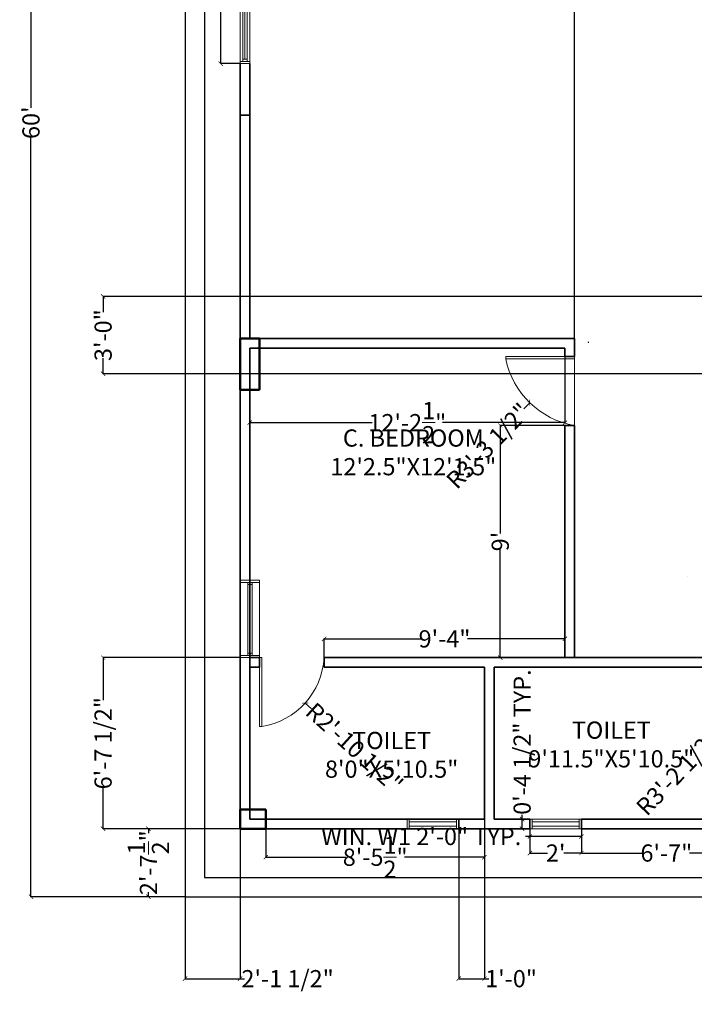
# Model space of a CAD drawing. Units: inches. Extents: x 490 to 1091, y 501 to 1322.
# Tile 1 of 5: x 490 to 804, y 501 to 959. Entities that reach past the tile are written whole.
import ezdxf

# ---------------------------------------------------------------- set-up
doc = ezdxf.new("R2010")
doc.units = ezdxf.units.IN
doc.header["$MEASUREMENT"] = 0
doc.linetypes.add('ACAD_ISO02W100', pattern=[15, 12, -3])
for name, color, linetype, lineweight in [('A-ANNO-DIMS', 2, 'Continuous', 18), ('A-ANNO-REFR', 8, 'Continuous', 13), ('A-AREA-IDEN', 7, 'Continuous', 25), ('A-COLS', 12, 'Continuous', 50), ('A-DOOR', 3, 'Continuous', 20), ('A-GLAZ', 4, 'Continuous', 18), ('A-WALL', 7, 'Continuous', 35), ('A-WALL-HIDN', 7, 'ACAD_ISO02W100', 18), ('C-PROP', 8, 'Continuous', 25)]:
    doc.layers.add(name, color=color, linetype=linetype, lineweight=lineweight)
doc.styles.get("Standard").update_dxf_attribs({"font": 'arial.ttf'})
doc.dimstyles.get("Standard").update_dxf_attribs({"dimtxt": 8, "dimasz": 2, "dimexe": 0.18, "dimexo": 0.0625, "dimgap": 0.09, "dimtad": 0, "dimdec": 1, "dimzin": 0, "dimdsep": 46, "dimlunit": 4, "dimtxsty": 'Standard', "dimblk": 'ARCHTICK', "dimcen": 0.09, "dimadec": 0, "dimazin": 0, "dimtfac": 1, "dimtdec": 1, "dimtofl": 0, "dimtmove": 0, "dimatfit": 3, "dimldrblk": 'ARCHTICK', "dimfxl": 1, "dimtolj": 1, "dimtzin": 0, "dimarcsym": 0})

# ---------------------------------------------------------------- blocks, each defined once
blk = doc.blocks.new('_ArchTick')
at = {"color": 0, "linetype": 'ByBlock', "const_width": 0.15}
blk.add_lwpolyline([(-0.5, -0.5), (0.5, 0.5)], dxfattribs=at)
blk = doc.blocks.new('*D4')
at = {"layer": 'A-ANNO-DIMS', "color": 0, "lineweight": -2, "transparency": 16777216}
for p, q in [((567.21, 1270.88), (495.41, 1270.88)), ((495.59, 1270.88), (495.59, 917.79)), ((495.59, 550.88), (495.59, 903.98)), ((567.21, 550.88), (495.41, 550.88))]:
    blk.add_line(p, q, dxfattribs=at)
at = {"layer": 'Defpoints', "color": 0, "transparency": 16777216}
for p in [(567.27, 1270.88), (495.59, 550.88), (567.27, 550.88)]:
    blk.add_point(p, dxfattribs=at)
at = {"layer": 'A-ANNO-DIMS', "color": 0, "lineweight": -2, "transparency": 16777216, "xscale": 2, "yscale": 2, "zscale": 2}
for p, rotation in [((495.59, 1270.88), 90), ((495.59, 550.88), 270)]:
    blk.add_blockref('_ArchTick', p, dxfattribs=dict(at, rotation=rotation))
at = {"layer": 'A-ANNO-DIMS', "color": 0, "transparency": 16777216, "insert": (495.59, 910.88), "char_height": 8, "attachment_point": 5, "rotation": 90}
blk.add_mtext("\\A1;60'", dxfattribs=at)
blk = doc.blocks.new('bfgbfhnfh')
for p, q in [((1236.93, 946.75), (1241.43, 946.75)), ((1236.93, 922.75), (1236.93, 946.75)), ((1236.93, 945.75), (1241.43, 945.75)), ((1238.18, 945.75), (1238.18, 923.75)), ((1240.18, 945.75), (1240.18, 923.75)), ((1241.43, 946.75), (1241.43, 922.75)), ((1241.43, 923.75), (1236.93, 923.75)), ((1241.43, 922.75), (1236.93, 922.75))]:
    blk.add_line(p, q)
blk = doc.blocks.new('bnfgfhvhm')
for p, q in [((1106.43, 1203.63), (1115.43, 1203.63)), ((1106.43, 1191.63), (1106.43, 1203.63)), ((1115.43, 1203.63), (1115.43, 1191.63)), ((1115.43, 1191.63), (1106.43, 1191.63))]:
    blk.add_line(p, q)
blk = doc.blocks.new('*D18')
at = {"layer": 'A-ANNO-DIMS', "color": 0, "lineweight": -2, "transparency": 16777216}
for p, q in [((751.67, 586.92), (751.67, 571.01)), ((830.67, 586.92), (830.67, 571.01)), ((751.67, 571.19), (780.42, 571.19)), ((830.67, 571.19), (801.91, 571.19))]:
    blk.add_line(p, q, dxfattribs=at)
at = {"layer": 'Defpoints', "color": 0, "transparency": 16777216}
for p in [(751.67, 586.98), (830.67, 586.98), (751.67, 571.19)]:
    blk.add_point(p, dxfattribs=at)
at = {"layer": 'A-ANNO-DIMS', "color": 0, "lineweight": -2, "transparency": 16777216, "xscale": 2, "yscale": 2, "zscale": 2, "rotation": 180}
blk.add_blockref('_ArchTick', (751.67, 571.19), dxfattribs=at)
at = {"layer": 'A-ANNO-DIMS', "color": 0, "lineweight": -2, "transparency": 16777216, "xscale": 2, "yscale": 2, "zscale": 2}
blk.add_blockref('_ArchTick', (830.67, 571.19), dxfattribs=at)
at = {"layer": 'A-ANNO-DIMS', "color": 0, "transparency": 16777216, "insert": (791.17, 571.19), "char_height": 8, "attachment_point": 5}
blk.add_mtext('\\A1;6\'-7"', dxfattribs=at)
blk = doc.blocks.new('*D19')
at = {"layer": 'A-ANNO-DIMS', "color": 0, "lineweight": -2, "transparency": 16777216}
for p, q in [((727.67, 582.42), (727.67, 571.01)), ((751.67, 582.42), (751.67, 571.01)), ((727.67, 571.19), (735.83, 571.19)), ((751.67, 571.19), (743.51, 571.19))]:
    blk.add_line(p, q, dxfattribs=at)
at = {"layer": 'Defpoints', "color": 0, "transparency": 16777216}
for p in [(727.67, 582.48), (751.67, 582.48), (751.67, 571.19)]:
    blk.add_point(p, dxfattribs=at)
at = {"layer": 'A-ANNO-DIMS', "color": 0, "lineweight": -2, "transparency": 16777216, "xscale": 2, "yscale": 2, "zscale": 2, "rotation": 180}
blk.add_blockref('_ArchTick', (727.67, 571.19), dxfattribs=at)
at = {"layer": 'A-ANNO-DIMS', "color": 0, "lineweight": -2, "transparency": 16777216, "xscale": 2, "yscale": 2, "zscale": 2}
blk.add_blockref('_ArchTick', (751.67, 571.19), dxfattribs=at)
at = {"layer": 'A-ANNO-DIMS', "color": 0, "transparency": 16777216, "insert": (739.67, 571.19), "char_height": 8, "attachment_point": 5}
blk.add_mtext("\\A1;2'", dxfattribs=at)
blk = doc.blocks.new('*D20')
at = {"layer": 'A-ANNO-DIMS', "color": 0, "lineweight": -2, "transparency": 16777216}
for p, q in [((604.87, 586.92), (604.87, 569.06)), ((706.57, 586.92), (706.57, 569.06)), ((604.87, 569.24), (642.07, 569.24)), ((706.57, 569.24), (669.37, 569.24))]:
    blk.add_line(p, q, dxfattribs=at)
at = {"layer": 'Defpoints', "color": 0, "transparency": 16777216}
for p in [(604.87, 586.98), (706.57, 586.98), (706.57, 569.24)]:
    blk.add_point(p, dxfattribs=at)
at = {"layer": 'A-ANNO-DIMS', "color": 0, "lineweight": -2, "transparency": 16777216, "xscale": 2, "yscale": 2, "zscale": 2, "rotation": 180}
blk.add_blockref('_ArchTick', (604.87, 569.24), dxfattribs=at)
at = {"layer": 'A-ANNO-DIMS', "color": 0, "lineweight": -2, "transparency": 16777216, "xscale": 2, "yscale": 2, "zscale": 2}
blk.add_blockref('_ArchTick', (706.57, 569.24), dxfattribs=at)
at = {"layer": 'A-ANNO-DIMS', "color": 0, "transparency": 16777216, "insert": (655.72, 569.24), "char_height": 8, "attachment_point": 5}
blk.add_mtext('\\A1;8\'-5{\\H1x;\\S1/2;}"', dxfattribs=at)
blk = doc.blocks.new('*D21')
at = {"layer": 'A-ANNO-DIMS', "color": 0, "lineweight": -2, "transparency": 16777216}
for p, q in [((631.97, 662.15), (631.97, 670.99)), ((631.97, 670.81), (677.25, 670.81)), ((743.97, 670.81), (698.69, 670.81)), ((743.97, 662.15), (743.97, 670.99))]:
    blk.add_line(p, q, dxfattribs=at)
at = {"layer": 'Defpoints', "color": 0, "transparency": 16777216}
for p in [(631.97, 670.81), (631.97, 662.08), (743.97, 662.08)]:
    blk.add_point(p, dxfattribs=at)
at = {"layer": 'A-ANNO-DIMS', "color": 0, "lineweight": -2, "transparency": 16777216, "xscale": 2, "yscale": 2, "zscale": 2, "rotation": 180}
blk.add_blockref('_ArchTick', (631.97, 670.81), dxfattribs=at)
at = {"layer": 'A-ANNO-DIMS', "color": 0, "lineweight": -2, "transparency": 16777216, "xscale": 2, "yscale": 2, "zscale": 2}
blk.add_blockref('_ArchTick', (743.97, 670.81), dxfattribs=at)
at = {"layer": 'A-ANNO-DIMS', "color": 0, "transparency": 16777216, "insert": (687.97, 670.81), "char_height": 8, "attachment_point": 5}
blk.add_mtext('\\A1;9\'-4"', dxfattribs=at)
blk = doc.blocks.new('ggnhgjgfjhgjjjjjjjj')
for p, q in [((597.37, 998.37), (592.87, 998.37)), ((592.87, 998.37), (592.87, 938.37)), ((597.37, 998.37), (592.87, 998.37)), ((597.37, 997.37), (592.87, 997.37)), ((594.12, 997.37), (594.12, 939.37)), ((596.12, 996.37), (594.12, 996.37)), ((595.12, 996.37), (595.12, 940.37)), ((596.12, 997.37), (596.12, 939.37)), ((597.37, 938.37), (597.37, 998.37)), ((592.87, 939.37), (597.37, 939.37)), ((594.12, 940.37), (596.12, 940.37)), ((597.37, 938.37), (592.87, 938.37)), ((592.87, 938.37), (597.37, 938.37))]:
    blk.add_line(p, q)
blk = doc.blocks.new('jcjg  bmvh')
for p, q in [((1232.66, 1066.6), (1223.66, 1066.6)), ((1223.66, 1066.6), (1223.66, 1042.6)), ((1232.66, 1042.6), (1232.66, 1066.6)), ((1223.66, 1042.6), (1232.66, 1042.6))]:
    blk.add_line(p, q)
blk = doc.blocks.new('fvbfbvc hbmh')
for p, q in [((1342.5, 1176.65), (1378.5, 1176.65)), ((1342.5, 1167.65), (1342.5, 1176.65)), ((1343.5, 1167.65), (1343.5, 1176.65)), ((1343.5, 1173.15), (1377.5, 1173.15)), ((1344.5, 1171.15), (1344.5, 1173.15)), ((1376.5, 1173.15), (1376.5, 1171.15)), ((1377.5, 1176.65), (1377.5, 1167.65)), ((1378.5, 1176.65), (1378.5, 1167.65)), ((1343.5, 1171.15), (1377.5, 1171.15)), ((1344.5, 1172.15), (1376.5, 1172.15)), ((1378.5, 1167.65), (1342.5, 1167.65))]:
    blk.add_line(p, q)
blk = doc.blocks.new('*D36')
at = {"layer": 'A-ANNO-DIMS', "color": 0, "lineweight": -2, "transparency": 16777216}
for p, q in [((592.81, 582.48), (550.06, 582.48)), ((550.24, 582.48), (550.24, 580.39)), ((567.21, 550.88), (550.06, 550.88)), ((550.24, 550.88), (550.24, 552.98))]:
    blk.add_line(p, q, dxfattribs=at)
at = {"layer": 'Defpoints', "color": 0, "transparency": 16777216}
for p in [(550.24, 582.48), (592.87, 582.48), (567.27, 550.88)]:
    blk.add_point(p, dxfattribs=at)
at = {"layer": 'A-ANNO-DIMS', "color": 0, "lineweight": -2, "transparency": 16777216, "xscale": 2, "yscale": 2, "zscale": 2}
for p, rotation in [((550.24, 582.48), 90), ((550.24, 550.88), 270)]:
    blk.add_blockref('_ArchTick', p, dxfattribs=dict(at, rotation=rotation))
at = {"layer": 'A-ANNO-DIMS', "color": 0, "transparency": 16777216, "insert": (550.24, 566.68), "char_height": 8, "attachment_point": 5, "rotation": 90}
blk.add_mtext('\\A1;2\'-7{\\H1x;\\S1/2;}"', dxfattribs=at)
blk = doc.blocks.new('*D38')
at = {"layer": 'A-ANNO-DIMS', "color": 0, "lineweight": -2, "transparency": 16777216}
for p, q in [((748.41, 770.08), (713.71, 770.08)), ((713.89, 770.08), (713.89, 719.86)), ((713.89, 662.08), (713.89, 712.31)), ((748.41, 662.08), (713.71, 662.08))]:
    blk.add_line(p, q, dxfattribs=at)
at = {"layer": 'Defpoints', "color": 0, "transparency": 16777216}
for p in [(748.47, 770.08), (713.89, 662.08), (748.47, 662.08)]:
    blk.add_point(p, dxfattribs=at)
at = {"layer": 'A-ANNO-DIMS', "color": 0, "lineweight": -2, "transparency": 16777216, "xscale": 2, "yscale": 2, "zscale": 2}
for p, rotation in [((713.89, 770.08), 90), ((713.89, 662.08), 270)]:
    blk.add_blockref('_ArchTick', p, dxfattribs=dict(at, rotation=rotation))
at = {"layer": 'A-ANNO-DIMS', "color": 0, "transparency": 16777216, "insert": (713.89, 716.08), "char_height": 8, "attachment_point": 5, "rotation": 90}
blk.add_mtext("\\A1;9'", dxfattribs=at)
blk = doc.blocks.new('*D39')
at = {"layer": 'A-ANNO-DIMS', "color": 0, "lineweight": -2, "transparency": 16777216}
for p, q in [((597.37, 806.02), (597.37, 771.19)), ((743.97, 806.02), (743.97, 771.19)), ((597.37, 771.37), (654.3, 771.37)), ((743.97, 771.37), (687.04, 771.37))]:
    blk.add_line(p, q, dxfattribs=at)
at = {"layer": 'Defpoints', "color": 0, "transparency": 16777216}
for p in [(597.37, 806.08), (743.97, 806.08), (743.97, 771.37)]:
    blk.add_point(p, dxfattribs=at)
at = {"layer": 'A-ANNO-DIMS', "color": 0, "lineweight": -2, "transparency": 16777216, "xscale": 2, "yscale": 2, "zscale": 2, "rotation": 180}
blk.add_blockref('_ArchTick', (597.37, 771.37), dxfattribs=at)
at = {"layer": 'A-ANNO-DIMS', "color": 0, "lineweight": -2, "transparency": 16777216, "xscale": 2, "yscale": 2, "zscale": 2}
blk.add_blockref('_ArchTick', (743.97, 771.37), dxfattribs=at)
at = {"layer": 'A-ANNO-DIMS', "color": 0, "transparency": 16777216, "insert": (670.67, 771.37), "char_height": 8, "attachment_point": 5}
blk.add_mtext('\\A1;12\'-2{\\H1x;\\S1/2;}"', dxfattribs=at)
blk = doc.blocks.new('DOOR-LEAF-32IN')
for p, q in [((-32, -1), (-32, 0)), ((-32, 0), (0, 0)), ((0, 0), (0, -1)), ((0, -1), (-32, -1))]:
    blk.add_line(p, q)
blk = doc.blocks.new('*D58')
at = {"layer": 'A-ANNO-DIMS', "color": 0, "lineweight": -2, "transparency": 16777216}
for p, q in [((727.67, 582.42), (727.67, 578.7)), ((751.67, 582.42), (751.67, 578.7)), ((727.67, 578.88), (725.67, 578.88)), ((751.67, 578.88), (727.67, 578.88))]:
    blk.add_line(p, q, dxfattribs=at)
at = {"layer": 'Defpoints', "color": 0, "transparency": 16777216}
for p in [(727.67, 582.48), (751.67, 582.48), (727.67, 578.88)]:
    blk.add_point(p, dxfattribs=at)
at = {"layer": 'A-ANNO-DIMS', "color": 0, "lineweight": -2, "transparency": 16777216, "xscale": 2, "yscale": 2, "zscale": 2, "rotation": 180}
blk.add_blockref('_ArchTick', (727.67, 578.88), dxfattribs=at)
at = {"layer": 'A-ANNO-DIMS', "color": 0, "lineweight": -2, "transparency": 16777216, "xscale": 2, "yscale": 2, "zscale": 2}
blk.add_blockref('_ArchTick', (751.67, 578.88), dxfattribs=at)
at = {"layer": 'A-ANNO-DIMS', "color": 0, "transparency": 16777216, "insert": (677.13, 578.88), "char_height": 8, "attachment_point": 5}
blk.add_mtext('\\A1;WIN. W1 2\'-0" TYP.', dxfattribs=at)
blk = doc.blocks.new('*D59')
at = {"layer": 'A-ANNO-DIMS', "color": 0, "lineweight": -2, "transparency": 16777216}
for p, q in [((727.61, 586.98), (723.89, 586.98)), ((724.07, 586.98), (724.07, 588.98)), ((724.07, 582.48), (724.07, 586.98)), ((727.61, 582.48), (723.89, 582.48))]:
    blk.add_line(p, q, dxfattribs=at)
at = {"layer": 'Defpoints', "color": 0, "transparency": 16777216}
for p in [(724.07, 586.98), (727.67, 586.98), (727.67, 582.48)]:
    blk.add_point(p, dxfattribs=at)
at = {"layer": 'A-ANNO-DIMS', "color": 0, "lineweight": -2, "transparency": 16777216, "xscale": 2, "yscale": 2, "zscale": 2}
for p, rotation in [((724.07, 586.98), 90), ((724.07, 582.48), 270)]:
    blk.add_blockref('_ArchTick', p, dxfattribs=dict(at, rotation=rotation))
at = {"layer": 'A-ANNO-DIMS', "color": 0, "transparency": 16777216, "insert": (724.07, 622.78), "char_height": 8, "attachment_point": 5, "rotation": 90}
blk.add_mtext('\\A1;0\'-4 1/2" TYP.', dxfattribs=at)
blk = doc.blocks.new('*D62')
at = {"layer": 'A-ANNO-DIMS', "color": 0, "lineweight": -2, "transparency": 16777216}
for p, q in [((583.87, 998.37), (583.87, 1000.37)), ((592.81, 998.37), (583.69, 998.37)), ((583.87, 938.37), (583.87, 998.37)), ((592.81, 938.37), (583.69, 938.37))]:
    blk.add_line(p, q, dxfattribs=at)
at = {"layer": 'Defpoints', "color": 0, "transparency": 16777216}
for p in [(583.87, 998.37), (592.87, 998.37), (592.87, 938.37)]:
    blk.add_point(p, dxfattribs=at)
at = {"layer": 'A-ANNO-DIMS', "color": 0, "lineweight": -2, "transparency": 16777216, "xscale": 2, "yscale": 2, "zscale": 2}
for p, rotation in [((583.87, 998.37), 90), ((583.87, 938.37), 270)]:
    blk.add_blockref('_ArchTick', p, dxfattribs=dict(at, rotation=rotation))
at = {"layer": 'A-ANNO-DIMS', "color": 0, "transparency": 16777216, "insert": (583.87, 1035.16), "char_height": 8, "attachment_point": 5, "rotation": 90}
blk.add_mtext('\\A1;WIN. W3 5\'-0"', dxfattribs=at)
blk = doc.blocks.new('*D66')
at = {"layer": 'A-ANNO-DIMS', "color": 0, "lineweight": -2, "transparency": 16777216}
for p, q in [((592.87, 582.42), (592.87, 512.57)), ((567.27, 550.82), (567.27, 512.57)), ((567.27, 512.75), (592.87, 512.75)), ((592.87, 512.75), (594.87, 512.75))]:
    blk.add_line(p, q, dxfattribs=at)
at = {"layer": 'Defpoints', "color": 0, "transparency": 16777216}
for p in [(592.87, 582.48), (567.27, 550.88), (592.87, 512.75)]:
    blk.add_point(p, dxfattribs=at)
at = {"layer": 'A-ANNO-DIMS', "color": 0, "lineweight": -2, "transparency": 16777216, "xscale": 2, "yscale": 2, "zscale": 2, "rotation": 180}
blk.add_blockref('_ArchTick', (567.27, 512.75), dxfattribs=at)
at = {"layer": 'A-ANNO-DIMS', "color": 0, "lineweight": -2, "transparency": 16777216, "xscale": 2, "yscale": 2, "zscale": 2}
blk.add_blockref('_ArchTick', (592.87, 512.75), dxfattribs=at)
at = {"layer": 'A-ANNO-DIMS', "color": 0, "transparency": 16777216, "insert": (614.98, 512.75), "char_height": 8, "attachment_point": 5}
blk.add_mtext('\\A1;2\'-1 1/2"', dxfattribs=at)
blk = doc.blocks.new('*D76')
at = {"layer": 'A-ANNO-DIMS', "color": 0, "lineweight": -2, "transparency": 16777216}
for p, q in [((748.47, 802.15), (748.47, 1309.19)), ((748.47, 1309.01), (775.72, 1309.01)), ((830.67, 1309.01), (803.42, 1309.01)), ((830.67, 794.15), (830.67, 1309.19))]:
    blk.add_line(p, q, dxfattribs=at)
at = {"layer": 'Defpoints', "color": 0, "transparency": 16777216}
for p in [(830.67, 1309.01), (748.47, 802.08), (830.67, 794.08)]:
    blk.add_point(p, dxfattribs=at)
at = {"layer": 'A-ANNO-DIMS', "color": 0, "lineweight": -2, "transparency": 16777216, "xscale": 2, "yscale": 2, "zscale": 2, "rotation": 180}
blk.add_blockref('_ArchTick', (748.47, 1309.01), dxfattribs=at)
at = {"layer": 'A-ANNO-DIMS', "color": 0, "lineweight": -2, "transparency": 16777216, "xscale": 2, "yscale": 2, "zscale": 2}
blk.add_blockref('_ArchTick', (830.67, 1309.01), dxfattribs=at)
at = {"layer": 'A-ANNO-DIMS', "color": 0, "transparency": 16777216, "insert": (789.57, 1309.01), "char_height": 8, "attachment_point": 5}
blk.add_mtext('\\A1;6\'-10"', dxfattribs=at)
blk = doc.blocks.new('*D77')
at = {"layer": 'A-ANNO-DIMS', "color": 0, "lineweight": -2, "transparency": 16777216}
for p, q in [((592.91, 662.08), (528.96, 662.08)), ((529.14, 662.08), (529.14, 642.35)), ((529.14, 582.48), (529.14, 602.22)), ((592.81, 582.48), (528.96, 582.48))]:
    blk.add_line(p, q, dxfattribs=at)
at = {"layer": 'Defpoints', "color": 0, "transparency": 16777216}
for p in [(529.14, 662.08), (592.97, 662.08), (592.87, 582.48)]:
    blk.add_point(p, dxfattribs=at)
at = {"layer": 'A-ANNO-DIMS', "color": 0, "lineweight": -2, "transparency": 16777216, "xscale": 2, "yscale": 2, "zscale": 2}
for p, rotation in [((529.14, 662.08), 90), ((529.14, 582.48), 270)]:
    blk.add_blockref('_ArchTick', p, dxfattribs=dict(at, rotation=rotation))
at = {"layer": 'A-ANNO-DIMS', "color": 0, "transparency": 16777216, "insert": (529.14, 622.28), "char_height": 8, "attachment_point": 5, "rotation": 90}
blk.add_mtext('\\A1;6\'-7 1/2"', dxfattribs=at)
blk = doc.blocks.new('*D78')
at = {"layer": 'A-ANNO-DIMS', "color": 0, "lineweight": -2, "transparency": 16777216}
for p, q in [((694.57, 586.92), (694.57, 512.57)), ((706.57, 586.92), (706.57, 512.57)), ((694.57, 512.75), (706.57, 512.75)), ((706.57, 512.75), (708.57, 512.75))]:
    blk.add_line(p, q, dxfattribs=at)
at = {"layer": 'Defpoints', "color": 0, "transparency": 16777216}
for p in [(694.57, 586.98), (706.57, 586.98), (706.57, 512.75)]:
    blk.add_point(p, dxfattribs=at)
at = {"layer": 'A-ANNO-DIMS', "color": 0, "lineweight": -2, "transparency": 16777216, "xscale": 2, "yscale": 2, "zscale": 2, "rotation": 180}
blk.add_blockref('_ArchTick', (694.57, 512.75), dxfattribs=at)
at = {"layer": 'A-ANNO-DIMS', "color": 0, "lineweight": -2, "transparency": 16777216, "xscale": 2, "yscale": 2, "zscale": 2}
blk.add_blockref('_ArchTick', (706.57, 512.75), dxfattribs=at)
at = {"layer": 'A-ANNO-DIMS', "color": 0, "transparency": 16777216, "insert": (718.92, 512.75), "char_height": 8, "attachment_point": 5}
blk.add_mtext('\\A1;1\'-0"', dxfattribs=at)
blk = doc.blocks.new('*D79')
at = {"layer": 'A-ANNO-DIMS', "color": 0, "lineweight": -2, "transparency": 16777216}
for p, q in [((830.61, 830.08), (528.96, 830.08)), ((529.14, 830.08), (529.14, 822.81)), ((529.14, 794.08), (529.14, 801.36)), ((830.61, 794.08), (528.96, 794.08))]:
    blk.add_line(p, q, dxfattribs=at)
at = {"layer": 'Defpoints', "color": 0, "transparency": 16777216}
for p in [(529.14, 830.08), (830.67, 830.08), (830.67, 794.08)]:
    blk.add_point(p, dxfattribs=at)
at = {"layer": 'A-ANNO-DIMS', "color": 0, "lineweight": -2, "transparency": 16777216, "xscale": 2, "yscale": 2, "zscale": 2}
for p, rotation in [((529.14, 830.08), 90), ((529.14, 794.08), 270)]:
    blk.add_blockref('_ArchTick', p, dxfattribs=dict(at, rotation=rotation))
at = {"layer": 'A-ANNO-DIMS', "color": 0, "transparency": 16777216, "insert": (529.14, 812.08), "char_height": 8, "attachment_point": 5, "rotation": 90}
blk.add_mtext('\\A1;3\'-0"', dxfattribs=at)
blk = doc.blocks.new('*D83')
at = {"layer": 'A-ANNO-DIMS', "color": 0, "lineweight": -2, "transparency": 16777216}
for p, q in [((754.87, 808.8), (755.05, 808.8)), ((754.96, 808.71), (754.96, 808.89)), ((724.86, 777.73), (727.64, 780.6))]:
    blk.add_line(p, q, dxfattribs=at)
at = {"layer": 'Defpoints', "color": 0, "transparency": 16777216}
for p in [(754.96, 808.8), (727.64, 780.6)]:
    blk.add_point(p, dxfattribs=at)
at = {"layer": 'A-ANNO-DIMS', "color": 0, "lineweight": -2, "transparency": 16777216, "xscale": 2, "yscale": 2, "zscale": 2, "rotation": 45.90870563316058}
blk.add_blockref('_ArchTick', (727.64, 780.6), dxfattribs=at)
at = {"layer": 'A-ANNO-DIMS', "color": 0, "transparency": 16777216, "insert": (708.25, 760.59), "char_height": 8, "attachment_point": 5, "rotation": 45.9087}
blk.add_mtext('\\A1;R3\'-3 1/2"', dxfattribs=at)
blk = doc.blocks.new('*D84')
at = {"layer": 'A-ANNO-DIMS', "color": 0, "lineweight": -2, "transparency": 16777216}
for p, q in [((842.73, 656.51), (842.91, 656.51)), ((842.82, 656.42), (842.82, 656.6)), ((813.15, 625.82), (815.93, 628.69))]:
    blk.add_line(p, q, dxfattribs=at)
at = {"layer": 'Defpoints', "color": 0, "transparency": 16777216}
for p in [(842.82, 656.51), (815.93, 628.69)]:
    blk.add_point(p, dxfattribs=at)
at = {"layer": 'A-ANNO-DIMS', "color": 0, "lineweight": -2, "transparency": 16777216, "xscale": 2, "yscale": 2, "zscale": 2, "rotation": 45.97167705914391}
blk.add_blockref('_ArchTick', (815.93, 628.69), dxfattribs=at)
at = {"layer": 'A-ANNO-DIMS', "color": 0, "transparency": 16777216, "insert": (796.55, 608.65), "char_height": 8, "attachment_point": 5, "rotation": 45.9717}
blk.add_mtext('\\A1;R3\'-2 1/2"', dxfattribs=at)
blk = doc.blocks.new('*D86')
at = {"layer": 'A-ANNO-DIMS', "color": 0, "lineweight": -2, "transparency": 16777216}
for p, q in [((597.7, 663.91), (597.7, 664.09)), ((597.61, 664), (597.79, 664)), ((626.1, 638.27), (623.13, 640.95))]:
    blk.add_line(p, q, dxfattribs=at)
at = {"layer": 'Defpoints', "color": 0, "transparency": 16777216}
for p in [(597.7, 664), (623.13, 640.95)]:
    blk.add_point(p, dxfattribs=at)
at = {"layer": 'A-ANNO-DIMS', "color": 0, "lineweight": -2, "transparency": 16777216, "xscale": 2, "yscale": 2, "zscale": 2, "rotation": 137.8160408924442}
blk.add_blockref('_ArchTick', (623.13, 640.95), dxfattribs=at)
at = {"layer": 'A-ANNO-DIMS', "color": 0, "transparency": 16777216, "insert": (646.09, 620.15), "char_height": 8, "attachment_point": 5, "rotation": 317.816}
blk.add_mtext('\\A1;R2\'-10 1/2"', dxfattribs=at)

msp = doc.modelspace()

# ---------------------------------------------------------------- linework, layer by layer
at = {"layer": 'A-ANNO-REFR'}
for p, q in [((801.21, 699.83), (801.21, 699.83)), ((706.57, 586.98), (706.57, 586.98))]:
    msp.add_line(p, q, dxfattribs=at)
at = {"layer": 'A-DOOR'}
msp.add_line((748.47, 801.08), (748.47, 770.08), dxfattribs=at)
for centre, radius, start, end in [((754.96, 808.8), 39.25, 191.3312, 260.4876), ((597.7, 664), 34.32, 278.829, 356.8021)]:
    msp.add_arc(centre, radius, start, end, dxfattribs=at)
at = {"layer": 'A-WALL'}
for p, q in [((592.87, 938.37), (592.87, 582.48)), ((597.37, 938.37), (597.37, 810.58)), ((597.37, 914.37), (592.87, 914.37)), ((597.37, 810.58), (748.47, 810.58)), ((597.37, 806.08), (743.97, 806.08)), ((597.37, 806.08), (597.37, 586.98)), ((743.97, 806.08), (743.97, 802.08)), ((748.47, 810.58), (748.47, 802.08)), ((743.97, 802.08), (748.47, 802.08)), ((743.97, 770.08), (748.47, 770.08)), ((743.97, 770.08), (743.97, 662.08)), ((748.47, 770.08), (748.47, 662.08)), ((597.37, 662.08), (601.97, 662.08)), ((601.97, 662.08), (601.97, 657.58)), ((631.97, 662.08), (631.97, 657.58)), ((631.97, 662.08), (706.57, 662.08)), ((706.57, 662.08), (830.67, 662.08)), ((597.37, 657.58), (601.97, 657.58)), ((631.97, 657.58), (706.57, 657.58)), ((706.57, 586.98), (706.57, 657.58)), ((711.07, 586.98), (711.07, 657.58)), ((711.07, 657.58), (830.67, 657.58)), ((597.37, 586.98), (706.57, 586.98)), ((706.57, 586.98), (694.57, 586.98)), ((694.57, 586.98), (694.57, 582.48)), ((711.07, 586.98), (727.67, 586.98)), ((727.67, 582.48), (727.67, 586.98)), ((751.67, 582.48), (751.67, 586.98)), ((751.67, 586.98), (830.67, 586.98)), ((727.67, 582.48), (592.87, 582.48)), ((1021.67, 582.48), (751.67, 582.48))]:
    msp.add_line(p, q, dxfattribs=at)
at = {"layer": 'A-WALL-HIDN'}
for p, q in [((597.37, 810.58), (592.87, 810.58)), ((727.67, 582.48), (727.67, 586.98))]:
    msp.add_line(p, q, dxfattribs=at)
at = {"layer": 'C-PROP'}
for p, q in [((567.27, 1270.88), (567.27, 550.88)), ((576.27, 1261.88), (576.27, 559.88)), ((576.27, 559.88), (1038.27, 559.88)), ((567.27, 550.88), (1047.27, 550.88))]:
    msp.add_line(p, q, dxfattribs=at)

# ---------------------------------------------------------------- block references
at = {"layer": 'A-COLS'}
msp.add_blockref('jcjg  bmvh', (-630.79, -256.01), dxfattribs=at)
at = {"layer": 'A-COLS', "rotation": 270}
msp.add_blockref('bnfgfhvhm', (-598.76, 1697.92), dxfattribs=at)
at = {"layer": 'A-DOOR'}
msp.add_blockref('DOOR-LEAF-32IN', (748.47, 802.08), dxfattribs=at)
at = {"layer": 'A-DOOR', "rotation": 89.9999999999996}
msp.add_blockref('DOOR-LEAF-32IN', (601.97, 662.08), dxfattribs=at)
at = {"layer": 'A-GLAZ'}
msp.add_blockref('ggnhgjgfjhgjjjjjjjj', (0, 0), dxfattribs=at)
for name, p, rotation in [('fvbfbvc hbmh', (-574.68, 2040.59), 270), ('bfgbfhnfh', (1617.32, -654.45), 90), ('bfgbfhnfh', (1674.42, -654.45), 90)]:
    msp.add_blockref(name, p, dxfattribs=dict(at, rotation=rotation))

# ---------------------------------------------------------------- texts
at = {"layer": 'A-AREA-IDEN', "char_height": 8, "attachment_point": 1}
for s, width, insert in [('\\pxqc;C. BEDROOM\\P12\'2.5"X12\'1.5"', 78.9731, (633.97, 768.22)), ('\\pxqc;TOILET\\P9\'11.5"X5\'10.5"', 71.8623, (729.64, 632.36)), ('\\pxqc;TOILET\\P8\'0"X5\'10.5"', 70.8665, (627.94, 627.54))]:
    msp.add_mtext_dynamic_manual_height_columns(s, width=width, gutter_width=40, heights=[0], dxfattribs=dict(at, insert=insert))

# ---------------------------------------------------------------- dimensions: what is measured, and where the dimension line sits
at = {"layer": 'A-ANNO-DIMS'}
for base, p1, p2, override, picture, middle in [((830.67, 1309.01), (748.47, 802.08), (830.67, 794.08), {"dimdec": 1, "dimlfac": 1, "dimrnd": 0, "dimzin": 1, "dimdsep": 46, "dimlunit": 4, "dimfrac": 2}, '*D76', (789.57, 1309.01)), ((743.97, 771.37), (597.37, 806.08), (743.97, 806.08), {"dimclrd": 0, "dimclre": 0, "dimclrt": 0}, '*D39', (670.67, 771.37)), ((631.97, 670.81), (743.97, 662.08), (631.97, 662.08), {"dimclrd": 0, "dimclre": 0, "dimclrt": 0}, '*D21', (687.97, 670.81)), ((706.57, 569.24), (604.87, 586.98), (706.57, 586.98), {"dimclrd": 0, "dimclre": 0, "dimclrt": 0}, '*D20', (655.72, 569.24)), ((706.57, 512.75), (694.57, 586.98), (706.57, 586.98), {"dimdec": 1, "dimlfac": 1, "dimrnd": 0, "dimzin": 1, "dimdsep": 46, "dimlunit": 4, "dimfrac": 2}, '*D78', (718.92, 512.75)), ((751.67, 571.19), (830.67, 586.98), (751.67, 586.98), {"dimclrd": 0, "dimclre": 0, "dimclrt": 0}, '*D18', (791.17, 571.19)), ((592.87, 512.75), (567.27, 550.88), (592.87, 582.48), {"dimdec": 1, "dimlfac": 1, "dimrnd": 0, "dimzin": 1, "dimdsep": 46, "dimlunit": 4, "dimfrac": 2}, '*D66', (614.98, 512.75)), ((751.67, 571.19), (727.67, 582.48), (751.67, 582.48), {"dimclrd": 0, "dimclre": 0, "dimclrt": 0}, '*D19', (739.67, 571.19))]:
    dim = msp.add_linear_dim(base=base, p1=p1, p2=p2, dimstyle='Standard', override=override, dxfattribs=at)
    dim.commit()
    dim.dimension.update_dxf_attribs({"geometry": picture, "text_midpoint": middle})
for base, p1, p2, override, picture, middle in [((495.59, 550.88), (567.27, 1270.88), (567.27, 550.88), {"dimclrd": 0, "dimclre": 0, "dimclrt": 0}, '*D4', (495.59, 910.88)), ((529.14, 830.08), (830.67, 794.08), (830.67, 830.08), {"dimdec": 1, "dimlfac": 1, "dimrnd": 0, "dimzin": 1, "dimdsep": 46, "dimlunit": 4, "dimfrac": 2}, '*D79', (529.14, 812.08)), ((713.89, 662.08), (748.47, 770.08), (748.47, 662.08), {"dimclrd": 0, "dimclre": 0, "dimclrt": 0}, '*D38', (713.89, 716.08)), ((529.14, 662.08), (592.87, 582.48), (592.97, 662.08), {"dimdec": 1, "dimlfac": 1, "dimrnd": 0, "dimzin": 1, "dimdsep": 46, "dimlunit": 4, "dimfrac": 2}, '*D77', (529.14, 622.28)), ((550.24, 582.48), (567.27, 550.88), (592.87, 582.48), {"dimclrd": 0, "dimclre": 0, "dimclrt": 0}, '*D36', (550.24, 566.68))]:
    dim = msp.add_linear_dim(base=base, p1=p1, p2=p2, angle=90, dimstyle='Standard', override=override, dxfattribs=at)
    dim.commit()
    dim.dimension.update_dxf_attribs({"geometry": picture, "text_midpoint": middle})
for base, p1, p2, angle, text, picture, middle in [((583.87, 998.37), (592.87, 938.37), (592.87, 998.37), 90, 'WIN. W3 <>', '*D62', (583.87, 1035.16)), ((724.07, 586.98), (727.67, 582.48), (727.67, 586.98), 90, '<> TYP.', '*D59', (724.07, 622.78)), ((727.67, 578.88), (751.67, 582.48), (727.67, 582.48), 180, 'WIN. W1 <> TYP.', '*D58', (677.13, 578.88))]:
    dim = msp.add_linear_dim(base=base, p1=p1, p2=p2, angle=angle, text=text, dimstyle='Standard', override={"dimdec": 1, "dimlfac": 1, "dimrnd": 0, "dimzin": 1, "dimdsep": 46, "dimlunit": 4, "dimfrac": 2}, dxfattribs=at)
    dim.commit()
    dim.dimension.update_dxf_attribs({"geometry": picture, "text_midpoint": middle})
for center, mpoint, picture, middle in [((754.96, 808.8), (727.64, 780.6), '*D83', (708.25, 760.59)), ((597.7, 664), (623.13, 640.95), '*D86', (646.09, 620.15)), ((842.82, 656.51), (815.93, 628.69), '*D84', (796.55, 608.65))]:
    dim = msp.add_radius_dim(center=center, mpoint=mpoint, dimstyle='Standard', override={"dimdec": 1, "dimlfac": 1, "dimrnd": 0, "dimzin": 1, "dimdsep": 46, "dimlunit": 4, "dimfrac": 2}, dxfattribs=at)
    dim.commit()
    dim.dimension.update_dxf_attribs({"geometry": picture, "text_midpoint": middle})

doc.saveas('drawing.dxf')
